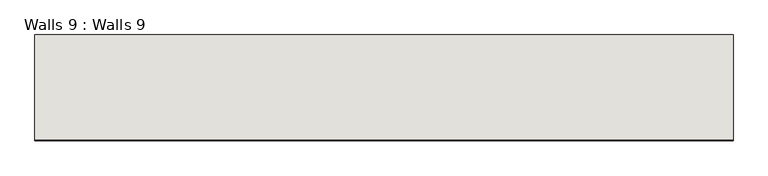
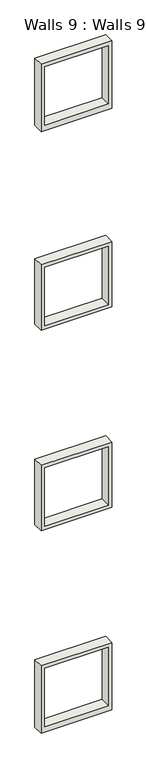
"""IFC4 building model written with IfcOpenShell, lengths in millimetres: wall geometry, Walls 9 : Walls 9."""

from ifc_helpers import new_model, si_unit, frame, origin, place, context, project, spatial, polyline, outline, extrude, source, transform, mapped, element, save


def walls_9_walls_9_93cd2fbd(model_context):
    return source(origin(), model_context, "Body", "SweptSolid", [
        extrude(outline(polyline([(11303.0, -4734.1569651), (11303.0, -5750.1569651), (10312.4, -5750.1569651), (10312.4, -4734.1569651), (11303.0, -4734.1569651)]), holes=[polyline([(11252.2, -4784.9569651), (10363.2, -4784.9569651), (10363.2, -5699.3569651), (11252.2, -5699.3569651), (11252.2, -4784.9569651)])]), frame((0.0, 2902.6055142, 0.0), z_axis=(0.0, 1.0, 0.0), x_axis=(0.0, 0.0, 1.0)), (0.0, 0.0, 1.0), 152.4),
        extrude(outline(polyline([(14351.0, -4734.1569651), (14351.0, -5750.1569651), (13330.6584417, -5750.1569651), (13330.6584417, -4734.1569651), (14351.0, -4734.1569651)]), holes=[polyline([(13411.2, -4784.9569651), (13411.2, -5699.3569651), (14300.2, -5699.3569651), (14300.2, -4784.9569651), (13411.2, -4784.9569651)])]), frame((0.0, 2902.6055142, 0.0), z_axis=(0.0, 1.0, 0.0), x_axis=(0.0, 0.0, 1.0)), (0.0, 0.0, 1.0), 152.4),
        extrude(outline(polyline([(8255.0, -4734.1569651), (8255.0, -5750.1569651), (7264.4, -5750.1569651), (7264.4, -4734.1569651), (8255.0, -4734.1569651)]), holes=[polyline([(8204.2, -4784.9569651), (7315.2, -4784.9569651), (7315.2, -5699.3569651), (8204.2, -5699.3569651), (8204.2, -4784.9569651)])]), frame((0.0, 2902.6055142, 0.0), z_axis=(0.0, 1.0, 0.0), x_axis=(0.0, 0.0, 1.0)), (0.0, 0.0, 1.0), 152.4),
        extrude(outline(polyline([(5207.0, -4734.1569651), (5207.0, -5750.1569651), (4186.6584417, -5750.1569651), (4186.6584417, -4734.1569651), (5207.0, -4734.1569651)]), holes=[polyline([(5156.2, -4784.9569651), (4267.2, -4784.9569651), (4267.2, -5699.3569651), (5156.2, -5699.3569651), (5156.2, -4784.9569651)])]), frame((0.0, 2902.6055142, 0.0), z_axis=(0.0, 1.0, 0.0), x_axis=(0.0, 0.0, 1.0)), (0.0, 0.0, 1.0), 152.4),
    ])


if __name__ == "__main__":
    model = new_model("IFC4")
    model_context = context("Model", 3, world=origin())
    ifc_project = project(units=[si_unit("LENGTHUNIT", "METRE", prefix="MILLI")], contexts=[model_context])
    site = spatial("IfcSite", under=ifc_project)
    building = spatial("IfcBuilding", under=site)
    placement = place(None, origin())
    walls_9_walls_9_shape = walls_9_walls_9_93cd2fbd(model_context)
    element("IfcWall", 1, ObjectType="Walls 9 : Walls 9", at=placement, inside=building, context=model_context, shape_type="MappedRepresentation", body=[
        mapped(walls_9_walls_9_shape, transform((0.0, 0.0, 0.0), x_axis=(1.0, 0.0, 0.0), y_axis=(0.0, 1.0, 0.0), z_axis=(0.0, 0.0, 1.0))),
    ])
    save(model, "model.ifc")

# Revit data of these elements
# Element 1 (IfcWall, "Walls 9 : Walls 9")
#   Materials on its faces: "Default Wall"
# Materials
#   "Default Wall": colour RGB 128 128 128, transparency 0, Cost = 0
